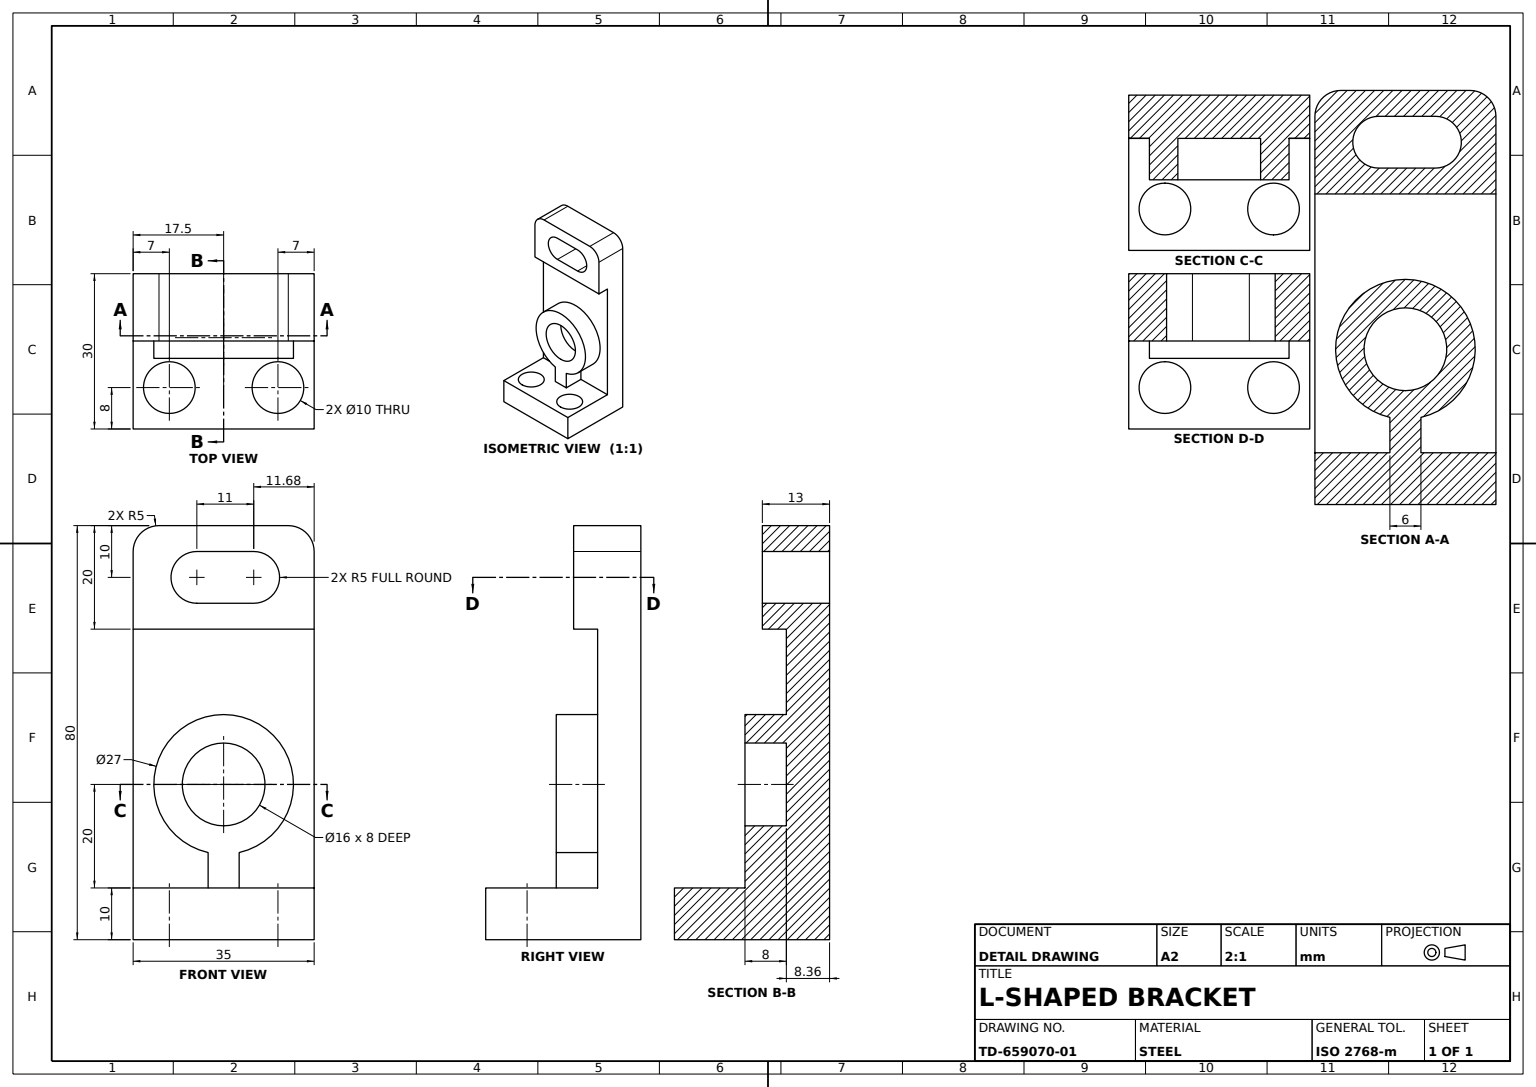
from build123d import *

# Parameters (mm, degrees)
BRACKET_PROFILE_SKETCH_W = 35
BRACKET_PROFILE_SKETCH_H = 80
BRACKET_BODY_DEPTH       = 30
SIDE_RELIEF_CUT_DEPTH    = 62.032778079
RING_BOSS_DEPTH          = 8
BOSS_BORE_SKETCH_R       = 8
BOSS_BORE_16_DEPTH       = 8
BASE_HOLES_SKETCH_R      = 5
BASE_HOLES_DEPTH         = 79.14249804
EDGE_FILLET_R5_R         = 5
TOP_SLOT_CUT_DEPTH       = 47.853495067


with BuildPart() as part:
    # Bracket Profile Sketch → Bracket Body (new body)
    with BuildSketch(Plane(origin=(0, 0, 0), x_dir=(0, 0, -1), z_dir=(1, 0, 0))):
        Rectangle(BRACKET_PROFILE_SKETCH_W, BRACKET_PROFILE_SKETCH_H)
    extrude(amount=BRACKET_BODY_DEPTH)

    # Side Relief Sketch → Side Relief Cut (cut, through all)
    with BuildSketch(Plane.XY.offset(17.5)):
        Polygon((13, 40), (13, 20), (8.358661264, 20), (8.358661264, -30), (30, -30), (30, 40), align=None)
    extrude(amount=-SIDE_RELIEF_CUT_DEPTH, mode=Mode.SUBTRACT)

    # Ring Boss Sketch → Ring Boss (add)
    with BuildSketch(Plane(origin=(8.358661264, 0, 0), x_dir=(0, 0, -1), z_dir=(1, 0, 0))):
        with BuildLine():
            Line((-3, -30), (3, -30))
            Line((3, -30), (3, -23.162446581))
            ThreePointArc((3, -23.162446581), (0, 3.5), (-3, -23.162446581))
            Line((-3, -23.162446581), (-3, -30))
        make_face()
    extrude(amount=RING_BOSS_DEPTH)

    # Boss Bore Sketch → Boss Bore Ø16 (cut)
    with BuildSketch(Plane(origin=(16.358661264, 0, 0), x_dir=(0, 0, -1), z_dir=(1, 0, 0))):
        with Locations(Location((0, -10, 0), (0, 0, 90))):
            Circle(BOSS_BORE_SKETCH_R)
    extrude(amount=-BOSS_BORE_16_DEPTH, mode=Mode.SUBTRACT)

    # Base Holes Sketch → Base Holes (cut, through all)
    with BuildSketch(Plane(origin=(0, -30, 0), x_dir=(1, 0, 0), z_dir=(0, 1, 0))):
        with Locations(Location((22, 10.5, 0), (0, 0, 180))):
            Circle(BASE_HOLES_SKETCH_R)
        with Locations((22, -10.5)):
            Circle(BASE_HOLES_SKETCH_R)
    extrude(amount=-BASE_HOLES_DEPTH, mode=Mode.SUBTRACT)

    # Edge Fillet R5
    edge_fillet_r5_edges = [part.edges().sort_by_distance(p)[0] for p in [
        (6.5, 40, 17.5),
        (6.5, 40, -17.5),
    ]]
    fillet(edge_fillet_r5_edges, radius=EDGE_FILLET_R5_R)

    # Top Slot Sketch → Top Slot Cut (cut, through all)
    with BuildSketch(Plane(origin=(13, 0, 0), x_dir=(0, 0, -1), z_dir=(1, 0, 0))):
        with BuildLine():
            Line((-5.180950854, 35), (5.819049146, 35))
            ThreePointArc((5.819049146, 35), (10.819049146, 30), (5.819049146, 25))
            Line((5.819049146, 25), (-5.180950854, 25))
            ThreePointArc((-5.180950854, 25), (-10.180950854, 30), (-5.180950854, 35))
        make_face()
    extrude(amount=-TOP_SLOT_CUT_DEPTH, mode=Mode.SUBTRACT)


solid = part.part
